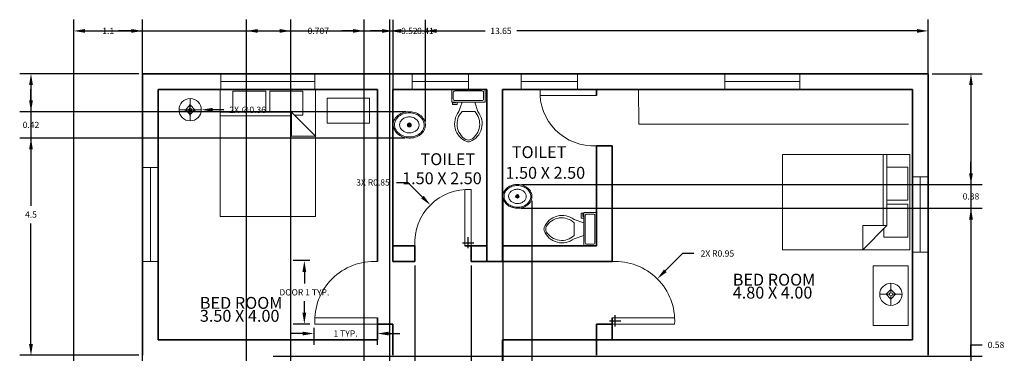
# Model space of a CAD drawing. Units: metres. Extents: x 180.3 to 196.1, y 135.7 to 166.1.
# Tile 5 of 5: x 180.3 to 196.1, y 160.8 to 166.1. Entities that reach past the tile are written whole.
import ezdxf

# ---------------------------------------------------------------- set-up
doc = ezdxf.new("R2010")
doc.units = ezdxf.units.M
doc.header["$MEASUREMENT"] = 0
for name, color, linetype, lineweight in [('A-ANNO-DIMS', 2, 'Continuous', 18), ('A-AREA-IDEN', 210, 'Continuous', 18), ('A-FLOR-CASE', 8, 'Continuous', 18), ('A-FLOR-FIXT', 9, 'Continuous', 18), ('A-FURN', 190, 'Continuous', 18), ('A-GLAZ', 130, 'Continuous', 18), ('A-GLAZ-VENT', 170, 'Continuous', 18), ('dim', 70, 'Continuous', 15), ('door', 240, 'Continuous', 18), ('wall', 50, 'Continuous', 35)]:
    doc.layers.add(name, color=color, linetype=linetype, lineweight=lineweight)
doc.styles.get("Standard").update_dxf_attribs({"font": 'arial.ttf', "height": 0.1})
doc.dimstyles.get("Standard").update_dxf_attribs({"dimtxt": 0.18, "dimasz": 0.18, "dimexe": 0.18, "dimexo": 0.0625, "dimgap": 0.09, "dimtad": 0, "dimtih": 1, "dimtoh": 1, "dimdec": 4, "dimzin": 0, "dimdsep": 46, "dimtxsty": 'Standard', "dimcen": 0.09, "dimadec": 0, "dimazin": 0, "dimtfac": 1, "dimtdec": 4, "dimtofl": 0, "dimtmove": 0, "dimatfit": 3, "dimfxl": 1, "dimtolj": 1, "dimtzin": 0, "dimarcsym": 0})

# ---------------------------------------------------------------- blocks, each defined once
blk = doc.blocks.new('Bed - Queen')
for p, q in [((0, -80.00003), (0, 0)), ((0, 0), (59.99999, 0)), ((59.99999, 0), (59.99999, -80.00003)), ((7.99999, -1.2), (28.79998, -1.2)), ((7.99999, -14.4), (7.99999, -1.2)), ((28.79998, -1.2), (28.79998, -14.4)), ((31.19999, -1.2), (51.99999, -1.2)), ((31.19999, -14.4), (31.19999, -1.2)), ((51.99999, -1.2), (51.99999, -16.4)), ((0, -14.4), (44.8, -14.4)), ((44.8, -16.8), (0, -16.8)), ((59.99999, -29.6), (44.8, -14.4)), ((44.8, -14.4), (44.8, -29.6)), ((51.99999, -16.4), (46.79936, -16.4)), ((44.8, -29.6), (59.99999, -29.6)), ((59.99999, -80.00003), (0, -80.00003))]:
    blk.add_line(p, q)
blk = doc.blocks.new('Toilet - top')
for p, q in [((9.5, -6), (9.5, -2)), ((-10, -8.5), (-8, -8.5)), ((-10, -9.5), (-10, -8.5)), ((-7, -9.5), (-10, -9.5)), ((-8, -8.5), (-8, -8)), ((-7, -8), (-7, -9.5)), ((-4, -8), (-6, -14)), ((4, -8), (6, -14)), ((4, -14), (-4, -14))]:
    blk.add_line(p, q)
blk.add_lwpolyline([(10.5, -8), (10.5, 0), (-10.5, 0), (-10.5, -8)], close=True)
for points in [[(-9.5, -2), (-9.5, -6)], [(8.5, -1), (-8.5, -1)], [(-8.5, -7), (8.5, -7)]]:
    blk.add_lwpolyline(points)
for centre, radius, start, end in [((-8.62, -1.88), 0.884, 81.8699, 188.1301), ((-8.62, -6.12), 0.884, 171.8699, 278.1301), ((8.62, -1.88), 0.884, 351.8699, 98.1301), ((8.62, -6.12), 0.884, 261.8699, 8.1301), ((3.52, -21.58), 12.17, 141.46911, 247.97143), ((4.2, -21.82), 11.33, 136.36773, 238.94682), ((-3.52, -21.58), 12.17, 292.02843, 38.53071), ((-4.2, -21.82), 11.33, 301.05301, 43.63209), ((0, -27.88), 4, 245.73182, 294.26817), ((0, -29), 4, 254.86053, 285.13947)]:
    blk.add_arc(centre, radius, start, end)
blk = doc.blocks.new('Sink - Oval top')
for p, q in [((-1, 0), (1, 0)), ((0, 1), (0, -1))]:
    blk.add_line(p, q)
for points in [[(-12.23, 0.39, 0.117634), (-11.46, -3.36, 0.104469), (-8.88, -6.8, 0.090016), (-5.08, -9.07, 0.08192), (-0.32, -10.02, 0.08192), (4.49, -9.38, 0.090016), (8.42, -7.36, 0.104469), (11.22, -4.09, 0.117634), (12.23, -0.39, 0.117634), (11.46, 3.36, 0.104469), (8.88, 6.8, 0.090016), (5.08, 9.07, 0.08192), (0.32, 10.02, 0.08192), (-4.49, 9.38, 0.090016), (-8.42, 7.36, 0.104469), (-11.22, 4.09, 0.117634)], [(-11.29, 0.16, 0.118622), (-10.52, -3.25, 0.104678), (-8.07, -6.36, 0.089562), (-4.54, -8.37, 0.081185), (-0.13, -9.15, 0.081185), (4.3, -8.49, 0.089562), (7.89, -6.58, 0.104678), (10.42, -3.55, 0.118622), (11.29, -0.16, 0.118622), (10.52, 3.25, 0.104678), (8.07, 6.36, 0.089562), (4.54, 8.37, 0.081185), (0.13, 9.15, 0.081185), (-4.3, 8.49, 0.089562), (-7.89, 6.58, 0.104678), (-10.42, 3.55, 0.118622)], [(-7.42, 0.08, 0.118283), (-6.91, -2.17, 0.104607), (-5.29, -4.21, 0.089718), (-2.97, -5.53, 0.081436), (-0.07, -6.04, 0.081436), (2.84, -5.59, 0.089718), (5.2, -4.33, 0.104607), (6.86, -2.32, 0.118283), (7.42, -0.08, 0.118283), (6.91, 2.17, 0.104607), (5.29, 4.21, 0.089718), (2.97, 5.53, 0.081436), (0.07, 6.04, 0.081436), (-2.84, 5.59, 0.089718), (-5.2, 4.33, 0.104607), (-6.86, 2.32, 0.118283)]]:
    blk.add_lwpolyline(points, format="xyb", close=True)
for radius in [1.5, 1]:
    blk.add_circle((0, 0), radius)
blk = doc.blocks.new('Lamp - Table')
for p, q in [((0, 7), (0, 1)), ((-1, 0), (-7, 0)), ((0, 3), (-3, 0)), ((-3, 0), (0, -3)), ((3, 0), (0, 3)), ((0, -3), (3, 0)), ((1, 0), (7, 0)), ((0, -1), (0, -7))]:
    blk.add_line(p, q)
for radius in [7, 1]:
    blk.add_circle((0, 0), radius)
blk = doc.blocks.new('DOOR-900')
for p, q in [((0.801, 0), (0.801, 0.9)), ((0.901, 0), (0.901, 0.9))]:
    blk.add_line(p, q)
blk.add_arc((0.851, 0.05), 0.851, 86.6335, 183.3665)
blk = doc.blocks.new('DOOR-1000')
for p, q in [((0, 0.1), (1, 0.1)), ((0, 0), (1, 0))]:
    blk.add_line(p, q)
blk.add_arc((0.05, 0.05), 0.951, 356.9872, 93.0128)
blk = doc.blocks.new('WIN-1500')
for p, q in [((0, 0.25), (0, 0)), ((1.5, 0.25), (1.5, 0)), ((1.5, 0.125), (0, 0.125))]:
    blk.add_line(p, q)
blk = doc.blocks.new('WIN-1200')
for p, q in [((0, 1.2), (0.25, 1.2)), ((0.125, 0), (0.125, 1.2)), ((0, 0), (0.25, 0))]:
    blk.add_line(p, q)
blk = doc.blocks.new('VENT-900')
for p, q in [((0, 0), (0, 0.25)), ((0.9, 0), (0.9, 0.25)), ((0.9, 0.125), (0, 0.125))]:
    blk.add_line(p, q)
blk = doc.blocks.new('*D19')
at = {"layer": 'A-ANNO-DIMS', "color": 0, "lineweight": -2, "transparency": 16777216}
for p, q in [((184.971, 162.262), (184.701, 162.262)), ((184.881, 162.082), (184.881, 161.897)), ((184.881, 161.428), (184.881, 161.613)), ((184.971, 161.248), (184.701, 161.248))]:
    blk.add_line(p, q, dxfattribs=at)
at = {"layer": 'A-ANNO-DIMS', "color": 0, "transparency": 16777216}
for points in [[(184.851, 162.082), (184.911, 162.082), (184.881, 162.262)], [(184.851, 161.428), (184.911, 161.428), (184.881, 161.248)]]:
    blk.add_solid(points, dxfattribs=at)
at = {"layer": 'Defpoints', "color": 0, "transparency": 16777216}
for p in [(184.881, 162.262), (185.033, 162.262), (185.033, 161.248)]:
    blk.add_point(p, dxfattribs=at)
at = {"layer": 'A-ANNO-DIMS', "color": 0, "transparency": 16777216, "insert": (184.881, 161.755), "char_height": 0.1, "attachment_point": 5}
blk.add_mtext('\\A1;DOOR 1 TYP.', dxfattribs=at)
blk = doc.blocks.new('*D20')
at = {"layer": 'A-ANNO-DIMS', "color": 0, "lineweight": -2, "transparency": 16777216}
for p, q in [((184.853, 161.096), (184.673, 161.096)), ((185.033, 161.185), (185.033, 160.916)), ((186.047, 161.185), (186.047, 160.916)), ((186.227, 161.096), (186.407, 161.096))]:
    blk.add_line(p, q, dxfattribs=at)
at = {"layer": 'A-ANNO-DIMS', "color": 0, "transparency": 16777216}
for points in [[(184.853, 161.126), (184.853, 161.066), (185.033, 161.096)], [(186.227, 161.126), (186.227, 161.066), (186.047, 161.096)]]:
    blk.add_solid(points, dxfattribs=at)
at = {"layer": 'Defpoints', "color": 0, "transparency": 16777216}
for p in [(185.033, 161.248), (186.047, 161.248), (185.033, 161.096)]:
    blk.add_point(p, dxfattribs=at)
at = {"layer": 'A-ANNO-DIMS', "color": 0, "transparency": 16777216, "insert": (185.54, 161.096), "char_height": 0.1, "attachment_point": 5}
blk.add_mtext('\\A1;1 TYP.', dxfattribs=at)
blk = doc.blocks.new('*D33')
at = {"layer": 'A-ANNO-DIMS', "color": 0, "lineweight": -2, "transparency": 16777216}
for p, q in [((181.197, 156.56), (181.197, 166.112)), ((194.847, 160.81), (194.847, 166.112)), ((181.377, 165.932), (187.768, 165.932)), ((194.667, 165.932), (188.277, 165.932))]:
    blk.add_line(p, q, dxfattribs=at)
at = {"layer": 'A-ANNO-DIMS', "color": 0, "transparency": 16777216}
for points in [[(181.377, 165.962), (181.377, 165.902), (181.197, 165.932)], [(194.667, 165.962), (194.667, 165.902), (194.847, 165.932)]]:
    blk.add_solid(points, dxfattribs=at)
at = {"layer": 'Defpoints', "color": 0, "transparency": 16777216}
for p in [(194.847, 165.932), (194.847, 160.748), (181.197, 156.498)]:
    blk.add_point(p, dxfattribs=at)
at = {"layer": 'A-ANNO-DIMS', "color": 0, "transparency": 16777216, "insert": (188.022, 165.932), "char_height": 0.1, "attachment_point": 5}
blk.add_mtext('\\A1;13.65', dxfattribs=at)
blk = doc.blocks.new('*D34')
at = {"layer": 'A-ANNO-DIMS', "color": 0, "lineweight": -2, "transparency": 16777216}
for p, q in [((194.91, 165.248), (195.711, 165.248)), ((195.531, 165.068), (195.531, 158.639)), ((195.531, 151.928), (195.531, 158.357)), ((193.61, 151.748), (195.711, 151.748))]:
    blk.add_line(p, q, dxfattribs=at)
at = {"layer": 'A-ANNO-DIMS', "color": 0, "transparency": 16777216}
for points in [[(195.501, 165.068), (195.561, 165.068), (195.531, 165.248)], [(195.501, 151.928), (195.561, 151.928), (195.531, 151.748)]]:
    blk.add_solid(points, dxfattribs=at)
at = {"layer": 'Defpoints', "color": 0, "transparency": 16777216}
for p in [(194.847, 165.248), (195.531, 165.248), (193.547, 151.748)]:
    blk.add_point(p, dxfattribs=at)
at = {"layer": 'A-ANNO-DIMS', "color": 0, "transparency": 16777216, "insert": (195.531, 158.498), "char_height": 0.1, "attachment_point": 5}
blk.add_mtext('\\A1;13.5', dxfattribs=at)
blk = doc.blocks.new('*D35')
at = {"layer": 'A-ANNO-DIMS', "color": 0, "lineweight": -2, "transparency": 16777216}
for p, q in [((181.197, 156.56), (181.197, 166.112)), ((182.297, 156.56), (182.297, 166.112)), ((181.377, 165.932), (181.581, 165.932)), ((182.117, 165.932), (181.914, 165.932))]:
    blk.add_line(p, q, dxfattribs=at)
at = {"layer": 'A-ANNO-DIMS', "color": 0, "transparency": 16777216}
for points in [[(181.377, 165.962), (181.377, 165.902), (181.197, 165.932)], [(182.117, 165.962), (182.117, 165.902), (182.297, 165.932)]]:
    blk.add_solid(points, dxfattribs=at)
at = {"layer": 'Defpoints', "color": 0, "transparency": 16777216}
for p in [(182.297, 165.932), (181.197, 156.498), (182.297, 156.498)]:
    blk.add_point(p, dxfattribs=at)
at = {"layer": 'A-ANNO-DIMS', "color": 0, "transparency": 16777216, "insert": (181.747, 165.932), "char_height": 0.1, "attachment_point": 5}
blk.add_mtext('\\A1;1.1', dxfattribs=at)
blk = doc.blocks.new('*D38')
at = {"layer": 'A-ANNO-DIMS', "color": 0, "lineweight": -2, "transparency": 16777216}
for p, q in [((182.235, 165.248), (180.334, 165.248)), ((180.514, 165.068), (180.514, 163.139)), ((180.514, 160.928), (180.514, 162.857)), ((182.235, 160.748), (180.334, 160.748))]:
    blk.add_line(p, q, dxfattribs=at)
at = {"layer": 'A-ANNO-DIMS', "color": 0, "transparency": 16777216}
for points in [[(180.484, 165.068), (180.544, 165.068), (180.514, 165.248)], [(180.484, 160.928), (180.544, 160.928), (180.514, 160.748)]]:
    blk.add_solid(points, dxfattribs=at)
at = {"layer": 'Defpoints', "color": 0, "transparency": 16777216}
for p in [(182.297, 165.248), (180.514, 160.748), (182.297, 160.748)]:
    blk.add_point(p, dxfattribs=at)
at = {"layer": 'A-ANNO-DIMS', "color": 0, "transparency": 16777216, "insert": (180.514, 162.998), "char_height": 0.1, "attachment_point": 5}
blk.add_mtext('\\A1;4.5', dxfattribs=at)
blk = doc.blocks.new('*D49')
at = {"layer": 'A-ANNO-DIMS', "color": 0, "lineweight": -2, "transparency": 16777216}
for p, q in [((180.513585, 160.927902), (180.513585, 161.107902)), ((182.234835, 160.747902), (180.333585, 160.747902)), ((182.234835, 160.397902), (180.333585, 160.397902)), ((180.513585, 160.217902), (180.513585, 160.037902))]:
    blk.add_line(p, q, dxfattribs=at)
at = {"layer": 'A-ANNO-DIMS', "color": 0, "transparency": 16777216}
for points in [[(180.483585, 160.927902), (180.543585, 160.927902), (180.513585, 160.747902)], [(180.483585, 160.217902), (180.543585, 160.217902), (180.513585, 160.397902)]]:
    blk.add_solid(points, dxfattribs=at)
at = {"layer": 'Defpoints', "color": 0, "transparency": 16777216}
for p in [(180.513585, 160.747902), (182.297335, 160.747902), (182.297335, 160.397902)]:
    blk.add_point(p, dxfattribs=at)
at = {"layer": 'A-ANNO-DIMS', "color": 0, "transparency": 16777216, "insert": (180.513585, 160.572902), "char_height": 0.1, "attachment_point": 5}
blk.add_mtext('\\A1;0.35', dxfattribs=at)
blk = doc.blocks.new('*D54')
at = {"layer": 'A-ANNO-DIMS', "color": 0, "lineweight": -2, "transparency": 16777216}
for p, q in [((186.647, 162.185), (186.647, 150.884)), ((187.547, 162.185), (187.547, 150.884)), ((186.827, 151.064), (187.367, 151.064)), ((187.547, 151.064), (187.727, 151.064))]:
    blk.add_line(p, q, dxfattribs=at)
at = {"layer": 'A-ANNO-DIMS', "color": 0, "transparency": 16777216}
for points in [[(186.827, 151.094), (186.827, 151.034), (186.647, 151.064)], [(187.367, 151.094), (187.367, 151.034), (187.547, 151.064)]]:
    blk.add_solid(points, dxfattribs=at)
at = {"layer": 'Defpoints', "color": 0, "transparency": 16777216}
for p in [(186.647, 162.248), (187.547, 162.248), (187.547, 151.064)]:
    blk.add_point(p, dxfattribs=at)
at = {"layer": 'A-ANNO-DIMS', "color": 0, "transparency": 16777216, "insert": (187.908, 151.064), "char_height": 0.1, "attachment_point": 5}
blk.add_mtext('\\A1;0.9', dxfattribs=at)
blk = doc.blocks.new('*D55')
at = {"layer": 'A-ANNO-DIMS', "color": 0, "lineweight": -2, "transparency": 16777216}
for p, q in [((186.300438, 164.501136), (186.300438, 166.111652)), ((186.815758, 164.484532), (186.815758, 166.111652)), ((186.120438, 165.931652), (185.940438, 165.931652)), ((186.995758, 165.931652), (187.175758, 165.931652))]:
    blk.add_line(p, q, dxfattribs=at)
at = {"layer": 'A-ANNO-DIMS', "color": 0, "transparency": 16777216}
for points in [[(186.120438, 165.961652), (186.120438, 165.901652), (186.300438, 165.931652)], [(186.995758, 165.961652), (186.995758, 165.901652), (186.815758, 165.931652)]]:
    blk.add_solid(points, dxfattribs=at)
at = {"layer": 'Defpoints', "color": 0, "transparency": 16777216}
for p in [(186.815758, 165.931652), (186.300438, 164.438636), (186.815758, 164.422032)]:
    blk.add_point(p, dxfattribs=at)
at = {"layer": 'A-ANNO-DIMS', "color": 0, "transparency": 16777216, "insert": (186.558098, 165.931652), "char_height": 0.1, "attachment_point": 5}
blk.add_mtext('\\A1;0.52', dxfattribs=at)
blk = doc.blocks.new('*D56')
at = {"layer": 'A-ANNO-DIMS', "color": 0, "lineweight": -2, "transparency": 16777216}
for p, q in [((180.514, 164.821), (180.514, 165.001)), ((186.502, 164.641), (180.334, 164.641)), ((186.489, 164.219), (180.334, 164.219)), ((180.514, 164.039), (180.514, 163.859))]:
    blk.add_line(p, q, dxfattribs=at)
at = {"layer": 'A-ANNO-DIMS', "color": 0, "transparency": 16777216}
for points in [[(180.484, 164.821), (180.544, 164.821), (180.514, 164.641)], [(180.484, 164.039), (180.544, 164.039), (180.514, 164.219)]]:
    blk.add_solid(points, dxfattribs=at)
at = {"layer": 'Defpoints', "color": 0, "transparency": 16777216}
for p in [(180.514, 164.641), (186.565, 164.641), (186.551, 164.219)]:
    blk.add_point(p, dxfattribs=at)
at = {"layer": 'A-ANNO-DIMS', "color": 0, "transparency": 16777216, "insert": (180.514, 164.43), "char_height": 0.1, "attachment_point": 5}
blk.add_mtext('\\A1;0.42', dxfattribs=at)
blk = doc.blocks.new('*D57')
at = {"layer": 'A-ANNO-DIMS', "color": 0, "lineweight": -2, "transparency": 16777216}
for p, q in [((188.053, 163.233), (188.053, 150.884)), ((188.517, 163.218), (188.517, 150.884)), ((187.873, 151.064), (187.693, 151.064)), ((188.697, 151.064), (188.877, 151.064))]:
    blk.add_line(p, q, dxfattribs=at)
at = {"layer": 'A-ANNO-DIMS', "color": 0, "transparency": 16777216}
for points in [[(187.873, 151.094), (187.873, 151.034), (188.053, 151.064)], [(188.697, 151.094), (188.697, 151.034), (188.517, 151.064)]]:
    blk.add_solid(points, dxfattribs=at)
at = {"layer": 'Defpoints', "color": 0, "transparency": 16777216}
for p in [(188.053, 163.295), (188.517, 163.28), (188.517, 151.064)]:
    blk.add_point(p, dxfattribs=at)
at = {"layer": 'A-ANNO-DIMS', "color": 0, "transparency": 16777216, "insert": (188.285, 151.064), "char_height": 0.1, "attachment_point": 5}
blk.add_mtext('\\A1;0.46', dxfattribs=at)
blk = doc.blocks.new('*D58')
at = {"layer": 'A-ANNO-DIMS', "color": 0, "lineweight": -2, "transparency": 16777216}
for p, q in [((195.531, 163.658), (195.531, 163.838)), ((188.353, 163.478), (195.711, 163.478)), ((188.341, 163.098), (195.711, 163.098)), ((195.531, 162.918), (195.531, 162.738))]:
    blk.add_line(p, q, dxfattribs=at)
at = {"layer": 'A-ANNO-DIMS', "color": 0, "transparency": 16777216}
for points in [[(195.501, 163.658), (195.561, 163.658), (195.531, 163.478)], [(195.501, 162.918), (195.561, 162.918), (195.531, 163.098)]]:
    blk.add_solid(points, dxfattribs=at)
at = {"layer": 'Defpoints', "color": 0, "transparency": 16777216}
for p in [(188.291, 163.478), (195.531, 163.478), (188.279, 163.098)]:
    blk.add_point(p, dxfattribs=at)
at = {"layer": 'A-ANNO-DIMS', "color": 0, "transparency": 16777216, "insert": (195.531, 163.288), "char_height": 0.1, "attachment_point": 5}
blk.add_mtext('\\A1;0.38', dxfattribs=at)
blk = doc.blocks.new('*D59')
at = {"layer": 'A-ANNO-DIMS', "color": 0, "lineweight": -2, "transparency": 16777216}
for p, q in [((183.958, 160.518), (183.958, 166.112)), ((184.665, 160.495), (184.665, 166.112)), ((184.138, 165.932), (184.485, 165.932)), ((184.665, 165.932), (184.845, 165.932))]:
    blk.add_line(p, q, dxfattribs=at)
at = {"layer": 'A-ANNO-DIMS', "color": 0, "transparency": 16777216}
for points in [[(184.138, 165.962), (184.138, 165.902), (183.958, 165.932)], [(184.485, 165.962), (184.485, 165.902), (184.665, 165.932)]]:
    blk.add_solid(points, dxfattribs=at)
at = {"layer": 'Defpoints', "color": 0, "transparency": 16777216}
for p in [(184.665, 165.932), (183.958, 160.456), (184.665, 160.433)]:
    blk.add_point(p, dxfattribs=at)
at = {"layer": 'A-ANNO-DIMS', "color": 0, "transparency": 16777216, "insert": (185.104, 165.932), "char_height": 0.1, "attachment_point": 5}
blk.add_mtext('\\A1;0.707', dxfattribs=at)
blk = doc.blocks.new('*D60')
at = {"layer": 'A-ANNO-DIMS', "color": 0, "lineweight": -2, "transparency": 16777216}
for p, q in [((195.531, 160.734), (195.531, 160.914)), ((195.531, 160.914), (195.711, 160.914)), ((184.383, 160.734), (195.711, 160.734)), ((195.531, 160.335), (195.531, 160.554)), ((184.365, 160.155), (195.711, 160.155))]:
    blk.add_line(p, q, dxfattribs=at)
at = {"layer": 'A-ANNO-DIMS', "color": 0, "transparency": 16777216}
for points in [[(195.501, 160.554), (195.561, 160.554), (195.531, 160.734)], [(195.501, 160.335), (195.561, 160.335), (195.531, 160.155)]]:
    blk.add_solid(points, dxfattribs=at)
at = {"layer": 'Defpoints', "color": 0, "transparency": 16777216}
for p in [(184.321, 160.734), (195.531, 160.734), (184.302, 160.155)]:
    blk.add_point(p, dxfattribs=at)
at = {"layer": 'A-ANNO-DIMS', "color": 0, "transparency": 16777216, "insert": (195.931, 160.914), "char_height": 0.1, "attachment_point": 5}
blk.add_mtext('\\A1;0.58', dxfattribs=at)
blk = doc.blocks.new('*D63')
at = {"layer": 'A-ANNO-DIMS', "color": 0, "lineweight": -2, "transparency": 16777216}
for p, q in [((185.838, 153.874), (185.838, 166.112)), ((186.245, 153.876), (186.245, 166.112)), ((185.658, 165.932), (185.478, 165.932)), ((186.425, 165.932), (186.605, 165.932))]:
    blk.add_line(p, q, dxfattribs=at)
at = {"layer": 'A-ANNO-DIMS', "color": 0, "transparency": 16777216}
for points in [[(185.658, 165.962), (185.658, 165.902), (185.838, 165.932)], [(186.425, 165.962), (186.425, 165.902), (186.245, 165.932)]]:
    blk.add_solid(points, dxfattribs=at)
at = {"layer": 'Defpoints', "color": 0, "transparency": 16777216}
for p in [(186.245, 165.932), (185.838, 153.811), (186.245, 153.813)]:
    blk.add_point(p, dxfattribs=at)
at = {"layer": 'A-ANNO-DIMS', "color": 0, "transparency": 16777216, "insert": (186.815, 165.932), "char_height": 0.1, "attachment_point": 5}
blk.add_mtext('\\A1;0.41', dxfattribs=at)
blk = doc.blocks.new('*D65')
at = {"layer": 'A-ANNO-DIMS', "color": 0, "lineweight": -2, "transparency": 16777216}
for p, q in [((183.057, 164.582), (183.057, 164.762)), ((182.967, 164.672), (183.147, 164.672)), ((183.595, 164.671), (183.415, 164.672))]:
    blk.add_line(p, q, dxfattribs=at)
at = {"layer": 'A-ANNO-DIMS', "color": 0, "transparency": 16777216}
blk.add_solid([(183.415, 164.702), (183.415, 164.642), (183.235, 164.672)], dxfattribs=at)
at = {"layer": 'Defpoints', "color": 0, "transparency": 16777216}
for p in [(182.88, 164.673), (183.235, 164.672)]:
    blk.add_point(p, dxfattribs=at)
at = {"layer": 'A-ANNO-DIMS', "color": 0, "transparency": 16777216, "insert": (183.975, 164.671), "char_height": 0.1, "attachment_point": 5}
blk.add_mtext('\\A1;2X ∅0.36', dxfattribs=at)
blk = doc.blocks.new('*D67')
at = {"layer": 'A-ANNO-DIMS', "color": 0, "lineweight": -2, "transparency": 16777216}
for p, q in [((190.923, 162.375), (190.647, 162.098)), ((191.103, 162.375), (190.923, 162.375)), ((189.757, 161.298), (189.937, 161.298)), ((189.847, 161.208), (189.847, 161.388))]:
    blk.add_line(p, q, dxfattribs=at)
at = {"layer": 'A-ANNO-DIMS', "color": 0, "transparency": 16777216}
blk.add_solid([(190.626, 162.119), (190.668, 162.077), (190.52, 161.971)], dxfattribs=at)
at = {"layer": 'Defpoints', "color": 0, "transparency": 16777216}
for p in [(190.52, 161.971), (189.847, 161.298)]:
    blk.add_point(p, dxfattribs=at)
at = {"layer": 'A-ANNO-DIMS', "color": 0, "transparency": 16777216, "insert": (191.48, 162.375), "char_height": 0.1, "attachment_point": 5}
blk.add_mtext('\\A1;2X R0.95', dxfattribs=at)
blk = doc.blocks.new('*D68')
at = {"layer": 'A-ANNO-DIMS', "color": 0, "lineweight": -2, "transparency": 16777216}
for p, q in [((186.354, 163.511), (186.534, 163.511)), ((186.534, 163.511), (186.768, 163.277)), ((187.407, 162.548), (187.587, 162.548)), ((187.497, 162.458), (187.497, 162.638))]:
    blk.add_line(p, q, dxfattribs=at)
at = {"layer": 'A-ANNO-DIMS', "color": 0, "transparency": 16777216}
blk.add_solid([(186.789, 163.298), (186.747, 163.256), (186.895, 163.15)], dxfattribs=at)
at = {"layer": 'Defpoints', "color": 0, "transparency": 16777216}
for p in [(186.895, 163.15), (187.497, 162.548)]:
    blk.add_point(p, dxfattribs=at)
at = {"layer": 'A-ANNO-DIMS', "color": 0, "transparency": 16777216, "insert": (185.978, 163.511), "char_height": 0.1, "attachment_point": 5}
blk.add_mtext('\\A1;3X R0.85', dxfattribs=at)

msp = doc.modelspace()

# ---------------------------------------------------------------- linework, layer by layer
at = {"layer": 'A-FLOR-CASE'}
for p, q in [((190.2203, 164.9979), (190.2253, 164.4417)), ((190.2253, 164.4417), (194.533, 164.4417))]:
    msp.add_line(p, q, dxfattribs=at)
at = {"layer": 'A-FURN'}
for points in [[(185.2442, 164.8591), (185.9244, 164.8591), (185.9244, 164.4595), (185.2442, 164.4595)], [(193.9704, 162.179), (194.5291, 162.179), (194.5291, 161.227), (193.9704, 161.227)]]:
    msp.add_lwpolyline(points, close=True, dxfattribs=at)
at = {"layer": 'wall'}
for p, q in [((182.2973, 165.2479), (186.2973, 165.2479)), ((182.2973, 160.7479), (182.2973, 165.2479)), ((186.2973, 165.2479), (188.0473, 165.2479)), ((188.0473, 165.2479), (189.7973, 165.2479)), ((189.7973, 165.2479), (194.8473, 165.2479)), ((194.8473, 160.7479), (194.8473, 165.2479)), ((182.5473, 164.9979), (186.0473, 164.9979)), ((182.5473, 160.9979), (182.5473, 164.9979)), ((186.0473, 164.9979), (186.0473, 162.2479)), ((186.2973, 164.9979), (186.2973, 162.2479)), ((186.2973, 164.9979), (187.7973, 164.9979)), ((187.7973, 164.9979), (187.7973, 162.4979)), ((188.0473, 164.9979), (188.0473, 162.2479)), ((188.0473, 164.9979), (189.5473, 164.9979)), ((189.5473, 164.9979), (189.5473, 164.8979)), ((189.5473, 164.9979), (189.7973, 164.9979)), ((189.7973, 164.9979), (194.5973, 164.9979)), ((194.5973, 160.9979), (194.5973, 164.9979)), ((189.5473, 164.0979), (189.7973, 164.0979)), ((189.5473, 164.0979), (189.5473, 162.4979)), ((189.7973, 164.0979), (189.7973, 162.2479)), ((186.2973, 162.4979), (186.6473, 162.4979)), ((186.6473, 162.4979), (186.6473, 162.2479)), ((187.4473, 162.4979), (187.7973, 162.4979)), ((187.5473, 162.4979), (187.5473, 162.2479)), ((187.7973, 162.4979), (187.7973, 162.2479)), ((188.0473, 162.4979), (189.5473, 162.4979)), ((186.2973, 162.2479), (186.6473, 162.2479)), ((187.5473, 162.2479), (188.0473, 162.2479)), ((188.0473, 162.2479), (189.7973, 162.2479)), ((189.7973, 162.2479), (189.5473, 162.2479)), ((186.0473, 161.3479), (186.0473, 160.9979)), ((186.0473, 161.2479), (186.2973, 161.2479)), ((186.2973, 161.2479), (186.2973, 160.7479)), ((189.5473, 160.7479), (189.5473, 161.2479)), ((189.7973, 161.2479), (189.5473, 161.2479)), ((189.7973, 160.9979), (189.7973, 161.3479)), ((186.0473, 160.9979), (182.5473, 160.9979)), ((188.0473, 160.9979), (188.0473, 160.4979)), ((189.5473, 160.9979), (188.0473, 160.9979)), ((189.7973, 160.9979), (189.5473, 160.9979)), ((189.7973, 160.9979), (194.5973, 160.9979))]:
    msp.add_line(p, q, dxfattribs=at)

# ---------------------------------------------------------------- block references
at = {"layer": 'A-FLOR-FIXT'}
for name, p, xscale, yscale, zscale in [('Toilet - top', (187.5017, 164.9979), 0.0254, 0.0254, 0.0254), ('Sink - Oval top', (186.5581, 164.4303), 0.0210614657168734, 0.0210614657168734, 0.0210614657168734), ('Sink - Oval top', (188.2848, 163.2878), 0.0189505256562516, 0.0189505256562516, 0.0189505256562516)]:
    msp.add_blockref(name, p, dxfattribs=dict(at, xscale=xscale, yscale=yscale, zscale=zscale))
at = {"layer": 'A-FLOR-FIXT', "xscale": 0.0254, "yscale": 0.0254, "zscale": 0.0254, "rotation": 270}
msp.add_blockref('Toilet - top', (189.5473, 162.7646), dxfattribs=at)
at = {"layer": 'A-FURN', "xscale": 0.0254, "yscale": 0.0254, "zscale": 0.0254}
for name, p in [('Bed - Queen', (183.5361, 164.9999)), ('Lamp - Table', (183.0574, 164.6723)), ('Lamp - Table', (194.2517, 161.7233))]:
    msp.add_blockref(name, p, dxfattribs=at)
at = {"layer": 'A-FURN', "xscale": 0.0254, "yscale": 0.0254, "zscale": 0.0254, "rotation": 270.0000000000009}
msp.add_blockref('Bed - Queen', (194.5534, 163.9586), dxfattribs=at)
at = {"layer": 'A-GLAZ'}
for name, p in [('WIN-1500', (183.547, 164.998)), ('WIN-1200', (194.597, 162.398))]:
    msp.add_blockref(name, p, dxfattribs=at)
for name, p, rotation in [('WIN-1200', (191.5974, 165.2482), 270.0000000000021), ('WIN-1500', (182.5472, 162.2476), 89.99999999999683)]:
    msp.add_blockref(name, p, dxfattribs=dict(at, rotation=rotation))
at = {"layer": 'A-GLAZ-VENT', "rotation": 180}
msp.add_blockref('VENT-900', (187.5021, 165.2478), dxfattribs=at)
at = {"layer": 'A-GLAZ-VENT'}
msp.add_blockref('VENT-900', (188.347, 164.998), dxfattribs=at)
at = {"layer": 'door', "rotation": 90.0000000000016}
msp.add_blockref('DOOR-900', (189.5472, 164.0966), dxfattribs=at)
at = {"layer": 'door'}
for name, p in [('DOOR-900', (186.646, 162.498)), ('DOOR-1000', (189.797, 161.248))]:
    msp.add_blockref(name, p, dxfattribs=at)
at = {"layer": 'door', "extrusion": (0, 0, -1), "zscale": -1}
msp.add_blockref('DOOR-1000', (-186.0477, 161.248), dxfattribs=at)

# ---------------------------------------------------------------- texts
at = {"layer": 'A-AREA-IDEN', "char_height": 0.19, "attachment_point": 1}
for s, width, insert in [('TOILET ', 0.900113, (188.1961, 164.0897)), ('TOILET ', 0.900113, (186.7376, 163.9772)), ('BED ROOM', 2.305817, (191.7254, 162.0518)), ('BED ROOM', 2.305817, (183.2119, 161.6812))]:
    msp.add_mtext_dynamic_manual_height_columns(s, width=width, gutter_width=1, heights=[0], dxfattribs=dict(at, insert=insert))
at = {"layer": 'dim', "char_height": 0.19, "attachment_point": 1}
for s, width, insert in [('1.50 X 2.50 ', 1.656653, (188.0952, 163.7595)), ('1.50 X 2.50 ', 1.656653, (186.4436, 163.6723)), ('4.80 X 4.00 ', 1.525312, (191.7254, 161.8449)), ('3.50 X 4.00', 1.675595, (183.2119, 161.4743))]:
    msp.add_mtext_dynamic_manual_height_columns(s, width=width, gutter_width=1, heights=[0], dxfattribs=dict(at, insert=insert))

# ---------------------------------------------------------------- dimensions: what is measured, and where the dimension line sits
at = {"layer": 'A-ANNO-DIMS'}
for base, p1, p2, override, picture, middle in [((194.8473, 165.9317), (181.1973, 156.4979), (194.8473, 160.7479), {"dimdec": 2, "dimlfac": 1, "dimrnd": 0, "dimzin": 0, "dimdsep": 46, "dimlunit": 2}, '*D33', (188.0223, 165.9317)), ((182.2973, 165.9317), (181.1973, 156.4979), (182.2973, 156.4979), {"dimdec": 1, "dimlfac": 1, "dimrnd": 0, "dimzin": 0, "dimdsep": 46, "dimlunit": 2}, '*D35', (181.7473, 165.9317)), ((184.6651, 165.9317), (183.958, 160.4556), (184.6651, 160.4329), {"dimdec": 3, "dimlfac": 1, "dimrnd": 0, "dimzin": 0, "dimdsep": 46, "dimlunit": 2}, '*D59', (185.1038, 165.9317)), ((186.2446, 165.9317), (185.8382, 153.8113), (186.2446, 153.8132), {"dimdec": 2, "dimlfac": 1, "dimrnd": 0, "dimzin": 0, "dimdsep": 46, "dimlunit": 2}, '*D63', (186.8148, 165.9317)), ((186.8158, 165.9317), (186.3004, 164.4386), (186.8158, 164.422), {"dimdec": 2, "dimlfac": 1, "dimrnd": 0, "dimzin": 0, "dimdsep": 46, "dimlunit": 2}, '*D55', (186.5581, 165.9317)), ((188.5166, 151.0642), (188.0529, 163.2953), (188.5166, 163.2803), {"dimdec": 2, "dimlfac": 1, "dimrnd": 0, "dimzin": 0, "dimdsep": 46, "dimlunit": 2}, '*D57', (188.2848, 151.0642)), ((187.5473, 151.0642), (186.6473, 162.2479), (187.5473, 162.2479), {"dimdec": 1, "dimlfac": 1, "dimrnd": 0, "dimzin": 0, "dimdsep": 46, "dimlunit": 2}, '*D54', (187.9085, 151.0642))]:
    dim = msp.add_linear_dim(base=base, p1=p1, p2=p2, dimstyle='Standard', override=override, dxfattribs=at)
    dim.commit()
    dim.dimension.update_dxf_attribs({"geometry": picture, "text_midpoint": middle})
for base, p1, p2, override, picture, middle in [((180.5136, 160.7479), (182.2973, 165.2479), (182.2973, 160.7479), {"dimdec": 1, "dimlfac": 1, "dimrnd": 0, "dimzin": 0, "dimdsep": 46, "dimlunit": 2}, '*D38', (180.5136, 162.9979)), ((195.5311, 165.2479), (193.5473, 151.7479), (194.8473, 165.2479), {"dimdec": 1, "dimlfac": 1, "dimrnd": 0, "dimzin": 0, "dimdsep": 46, "dimlunit": 2}, '*D34', (195.5311, 158.4979)), ((180.5136, 164.6413), (186.5513, 164.2194), (186.5649, 164.6413), {"dimdec": 2, "dimlfac": 1, "dimrnd": 0, "dimzin": 0, "dimdsep": 46, "dimlunit": 2}, '*D56', (180.5136, 164.4303)), ((195.5311, 163.4776), (188.2786, 163.098), (188.2909, 163.4776), {"dimdec": 2, "dimlfac": 1, "dimrnd": 0, "dimzin": 0, "dimdsep": 46, "dimlunit": 2}, '*D58', (195.5311, 163.2878)), ((180.5136, 160.7479), (182.2973, 160.3979), (182.2973, 160.7479), {"dimdec": 2, "dimlfac": 1, "dimrnd": 0, "dimzin": 0, "dimdsep": 46, "dimlunit": 2}, '*D49', (180.5136, 160.5729)), ((195.5311, 160.7337), (184.3022, 160.1548), (184.3209, 160.7337), {"dimdec": 2, "dimlfac": 1, "dimrnd": 0, "dimzin": 0, "dimdsep": 46, "dimlunit": 2}, '*D60', (195.9311, 160.9137))]:
    dim = msp.add_linear_dim(base=base, p1=p1, p2=p2, angle=90, dimstyle='Standard', override=override, dxfattribs=at)
    dim.commit()
    dim.dimension.update_dxf_attribs({"geometry": picture, "text_midpoint": middle})
dim = msp.add_diameter_dim_2p(p1=(182.8796, 164.6725), p2=(183.2352, 164.672), text='2X <>', dimstyle='Standard', override={"dimdec": 2, "dimlfac": 1, "dimrnd": 0, "dimzin": 0, "dimdsep": 46, "dimlunit": 2}, dxfattribs=at)
dim.commit()
dim.dimension.update_dxf_attribs({"geometry": '*D65', "text_midpoint": (183.5952, 164.6715), "dimtype": 163})
for center, mpoint, text, picture, middle in [((187.4973, 162.5479), (186.8951, 163.1499), '3X <>', '*D68', (185.9783, 163.511)), ((189.8473, 161.2979), (190.5198, 161.9708), '2X <>', '*D67', (191.4797, 162.3745))]:
    dim = msp.add_radius_dim(center=center, mpoint=mpoint, text=text, dimstyle='Standard', override={"dimdec": 2, "dimlfac": 1, "dimrnd": 0, "dimzin": 0, "dimdsep": 46, "dimlunit": 2}, dxfattribs=at)
    dim.commit()
    dim.dimension.update_dxf_attribs({"geometry": picture, "text_midpoint": middle, "dimtype": 164})
for base, p1, p2, angle, text, picture, middle in [((184.881, 162.2621), (185.0332, 161.2479), (185.0332, 162.2621), 90, 'DOOR <> TYP.', '*D19', (184.881, 161.755)), ((185.0332, 161.0958), (186.0473, 161.2479), (185.0332, 161.2479), 180, '<> TYP.', '*D20', (185.5402, 161.0958))]:
    dim = msp.add_linear_dim(base=base, p1=p1, p2=p2, angle=angle, text=text, dimstyle='Standard', override={"dimdec": 0, "dimlfac": 1, "dimrnd": 0, "dimzin": 0, "dimdsep": 46, "dimlunit": 2}, dxfattribs=at)
    dim.commit()
    dim.dimension.update_dxf_attribs({"geometry": picture, "text_midpoint": middle})

doc.saveas('drawing.dxf')
